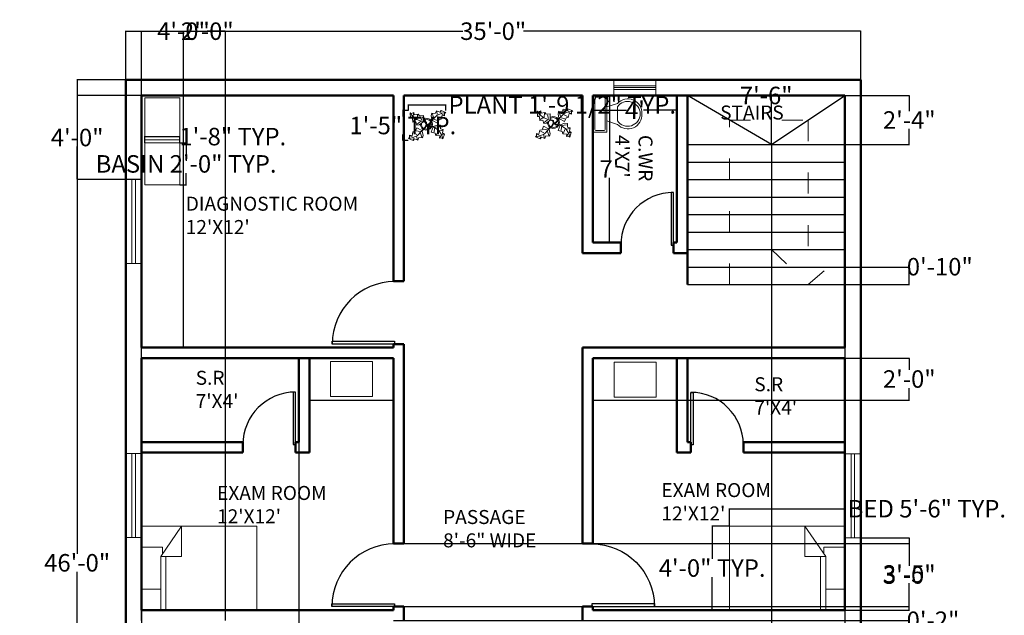
# Model space of a CAD drawing. Units: inches. Extents: x 69 to 644, y 258 to 887.
# Tile 3 of 3: x 82 to 644, y 546 to 887. Entities that reach past the tile are written whole.
import ezdxf

# ---------------------------------------------------------------- set-up
doc = ezdxf.new("R2010")
doc.units = ezdxf.units.IN
doc.header["$MEASUREMENT"] = 0
doc.linetypes.add('ACAD_ISO03W100', pattern=[30, 12, -18])
for name, color, linetype, lineweight in [('A-ANNO-DIMS', 2, 'Continuous', 18), ('A-AREA-IDEN', 7, 'Continuous', 25), ('A-DOOR', 4, 'Continuous', 25), ('A-EQPM-MED', 8, 'Continuous', 20), ('A-FLOR-CASE', 8, 'Continuous', 25), ('A-FLOR-FIXT', 9, 'Continuous', 18), ('A-FLOR-STRS', 7, 'Continuous', 25), ('A-FLOR-STRS-PATH', 7, 'ACAD_ISO03W100', 18), ('A-GLAZ', 4, 'Continuous', 18), ('A-WALL', 7, 'Continuous', 50), ('PLANT', 3, 'Continuous', 13)]:
    doc.layers.add(name, color=color, linetype=linetype, lineweight=lineweight)
doc.styles.get("Standard").update_dxf_attribs({"font": 'arial.ttf'})
doc.dimstyles.get("Standard").update_dxf_attribs({"dimtxt": 10, "dimasz": 0.18, "dimexe": 0.18, "dimexo": 0.0625, "dimgap": 0.09, "dimtad": 0, "dimtih": 1, "dimtoh": 1, "dimdec": 0, "dimzin": 0, "dimdsep": 46, "dimlunit": 3, "dimtxsty": 'Standard', "dimcen": 0.09, "dimadec": 0, "dimazin": 0, "dimtfac": 1, "dimtdec": 0, "dimtofl": 0, "dimtmove": 0, "dimatfit": 3, "dimfxl": 1, "dimtolj": 1, "dimtzin": 0, "dimarcsym": 0})

# ---------------------------------------------------------------- blocks, each defined once
blk = doc.blocks.new('SINGLE BED')
for p, q in [((0, 0), (0, -66)), ((48, 0), (0, 0)), ((12, 0), (12, -11)), ((36, -12), (36, 0)), ((48, -66), (48, 0)), ((0, -11), (30.52, -11)), ((30.52, -11), (48, -22.84)), ((30.52, -22.84), (30.52, -11)), ((0, -14), (30.52, -14)), ((31.99, -12), (36, -12)), ((48, -22.84), (30.52, -22.84)), ((0, -66), (48, -66))]:
    blk.add_line(p, q)
blk = doc.blocks.new('Plant - Rubber or Philodendron')
for p, q in [((-16.2005, 11.4774), (-13.9899, 8.1064)), ((-16.2005, 11.4774), (-14.8639, 10.7964)), ((-16.0159, 6.3329), (-16.2005, 11.4774)), ((-14.8639, 10.7964), (-12.6195, 11.8975)), ((-13.3174, 8.325), (-13.0735, 11.0065)), ((-12.6195, 11.8975), (-12.1909, 9.4345)), ((-12.1909, 9.4345), (-8.3829, 10.3)), ((-8.3829, 10.3), (-7.0549, 8.501)), ((4.6914, 8.8812), (5.3859, 11.2828)), ((5.3859, 11.2828), (8.8871, 10.7908)), ((5.9878, 10.4842), (7.1971, 6.3869)), ((8.8871, 10.7908), (9.9809, 13.4933)), ((9.9809, 13.4933), (13.3837, 12.301)), ((15.3859, 11.3055), (10.3916, 8.7942)), ((10.5828, 12.6946), (10.8893, 9.7953)), ((13.3837, 12.301), (14.68, 13.9039)), ((14.5816, 13.2037), (14.3848, 11.8033)), ((14.68, 13.9039), (19.3848, 11.8146)), ((15.2875, 10.6053), (17.5907, 9.2105)), ((19.3848, 11.8146), (15.3859, 11.3055)), ((19.3848, 11.8146), (18.1868, 10.9119)), ((18.1868, 10.9119), (18.1925, 8.4119)), ((-14.0069, 5.8704), (-16.0159, 6.3329)), ((-15.3434, 6.5514), (-13.9984, 6.9884)), ((-13.5868, 2.2894), (-14.0069, 5.8704)), ((-13.9899, 8.1064), (-9.5434, 4.7185)), ((-10.6784, 2.491), (-13.5868, 2.2894)), ((-13.1329, 3.1804), (-10.6614, 4.727)), ((-9.5858, -0.8715), (-10.6784, 2.491)), ((-9.5434, 4.7185), (-4.1917, 2.9888)), ((-9.1318, 0.0195), (-5.9793, 2.9025)), ((-8.8369, 9.409), (-9.0894, 5.6095)), ((-7.1228, -0.443), (-3.5248, 2.2131)), ((-7.0549, 8.501), (-3.0284, 8.6941)), ((-4.8529, 4.012), (-5.7184, 7.82)), ((-3.5248, 2.2131), (-3.3011, 2.4355)), ((-3.3011, 2.4355), (-0.5306, 1.7947)), ((-3.0284, 8.6941), (-3.0709, 3.1041)), ((-3.0709, 3.1041), (0.0797, 2.3163)), ((-0.5306, 1.7947), (-0.2255, -0.5527)), ((-0.5306, 1.7947), (-0.5306, 1.7947)), ((0.0797, 2.3163), (0.4866, -0.031)), ((0.4866, -0.031), (2.1141, 0.2298)), ((2.1141, 0.2298), (5.4346, 3.9146)), ((6.1032, 3.6844), (2.8262, -0.031)), ((4.6914, 8.8812), (5.5014, 4.4831)), ((5.4346, 3.9146), (5.5014, 4.4831)), ((11.1089, 1.1958), (6.1032, 3.6844)), ((10.3916, 8.7942), (6.2847, 4.4028)), ((7.7005, 4.8881), (11.5025, 3.9967)), ((14.2977, 6.1031), (10.9934, 7.9956)), ((12.7005, 4.8994), (11.1089, 1.1958)), ((14.8995, 5.3044), (12.7005, 4.8994)), ((15.7909, 9.1065), (14.8995, 5.3044)), ((18.1925, 8.4119), (15.7909, 9.1065)), ((-14.4141, -11.4699), (-13.5228, -7.6679)), ((-13.5228, -7.6679), (-11.3237, -7.2629)), ((-12.921, -8.4665), (-9.6166, -10.359)), ((-11.3237, -7.2629), (-9.7321, -3.5593)), ((-6.3237, -7.2516), (-10.1257, -6.3602)), ((-9.7321, -3.5593), (-4.7264, -6.0479)), ((-7.1228, -0.443), (-9.5858, -0.8715)), ((-9.0148, -11.1577), (-4.9047, -6.8122)), ((-4.611, -12.8477), (-5.8203, -8.7504)), ((-2.019, -3.6148), (-4.7264, -6.0479)), ((-4.1246, -6.8466), (-4.0579, -6.2781)), ((-3.3146, -11.2447), (-4.1246, -6.8466)), ((-4.0579, -6.2781), (-0.9375, -3.1608)), ((-2.019, -3.6148), (-0.2255, -0.5527)), ((-0.9375, -3.1608), (0.5883, -0.8135)), ((0.5883, -0.8135), (2.2447, -2.0916)), ((2.8262, -0.031), (1.3003, -0.5527)), ((1.3003, -0.5527), (2.4193, -1.4655)), ((2.2447, -2.0916), (6.7108, -2.6626)), ((2.4193, -1.4655), (6.895, -2.1175)), ((4.943, -7.9659), (6.7108, -2.6626)), ((8.8321, -9.0266), (4.943, -7.9659)), ((11.6605, -0.5413), (6.895, -2.1175)), ((12.3677, -6.1981), (7.219, -2.6772)), ((8.125, -4.0768), (7.7715, -7.9659)), ((8.3544, -2.7453), (13.1973, -2.1704)), ((9.5392, -11.1479), (8.8321, -9.0266)), ((10.2463, -10.4408), (11.6605, -6.9053)), ((11.6605, -0.5413), (14.1354, -0.8948)), ((15.5496, -10.7943), (12.3677, -6.1981)), ((16.2567, -5.8446), (13.4283, -6.5517)), ((14.1354, -0.8948), (14.1354, -4.4304)), ((14.1354, -4.4304), (16.9638, -5.1375)), ((17.3174, -9.7337), (15.9032, -9.7337)), ((16.9638, -5.1375), (16.2567, -8.673)), ((16.2567, -8.673), (18.0245, -9.7337)), ((18.0245, -9.7337), (16.6103, -14.6834)), ((-18.008, -14.1781), (-16.8101, -13.2754)), ((-18.008, -14.1781), (-14.0091, -13.669)), ((-13.3032, -16.2674), (-18.008, -14.1781)), ((-16.8157, -10.7754), (-14.4141, -11.4699)), ((-16.8101, -13.2754), (-16.8157, -10.7754)), ((-13.9107, -12.9688), (-16.2139, -11.574)), ((-14.0091, -13.669), (-9.0148, -11.1577)), ((-12.0069, -14.6645), (-13.3032, -16.2674)), ((-13.2048, -15.5672), (-13.008, -14.1668)), ((-8.6042, -15.8568), (-12.0069, -14.6645)), ((-9.206, -15.0581), (-9.5126, -12.1588)), ((-7.5103, -13.1543), (-8.6042, -15.8568)), ((-4.0092, -13.6463), (-7.5103, -13.1543)), ((-3.3146, -11.2447), (-4.0092, -13.6463)), ((13.4283, -11.5015), (9.5392, -11.1479)), ((13.0748, -13.9763), (13.4283, -11.5015)), ((15.5496, -13.6228), (13.0748, -13.9763)), ((14.8425, -10.7943), (13.7819, -13.2692)), ((16.6103, -14.6834), (15.5496, -10.7943)), ((16.6103, -14.6834), (15.5496, -13.6228))]:
    blk.add_line(p, q)
for centre, radius, start, end in [((0.0308, 0.1664), 6, 178.6147, 235.1169), ((0.0308, 0.1664), 5, 168.1647, 238.6725), ((0, 0), 6.1275, 34.37569, 120.1028), ((-0.0601, -0.2075), 5.2461, 33.82192, 124.9414), ((-0.2664, 0.1682), 5.2775, 338.4094, 20.03007), ((-0.098, 0.1364), 6.1288, 341.2017, 26.09184), ((-0.0234, 0.3825), 6.1492, 242.5812, 331.2714), ((-0.1102, 0.4886), 5.2883, 247.3711, 327.472)]:
    blk.add_arc(centre, radius, start, end)
blk = doc.blocks.new('*U14')
for p, q in [((0, 0), (0, -6)), ((40, 0), (40, -6))]:
    blk.add_line(p, q)
blk.add_lwpolyline([(0, 0), (0, 40), (1.75, 40), (1.75, 0)], close=True)
blk.add_arc((0, 0), 40, 0, 90)
blk = doc.blocks.new('*U15')
for p, q in [((0, 0), (0, -6)), ((-40, 0), (-40, -6))]:
    blk.add_line(p, q)
blk.add_lwpolyline([(0, 0), (0, 40), (-1.75, 40), (-1.75, 0)], close=True)
blk.add_arc((0, 0), 40, 90, 180)
blk = doc.blocks.new('*U17')
for p, q in [((9.5, -6), (9.5, -2)), ((-10, -8.5), (-8, -8.5)), ((-10, -9.5), (-10, -8.5)), ((-7, -9.5), (-10, -9.5)), ((-8, -8.5), (-8, -8)), ((-7, -8), (-7, -9.5)), ((-4, -8), (-6, -14)), ((4, -8), (6, -14)), ((4, -14), (-4, -14))]:
    blk.add_line(p, q)
blk.add_lwpolyline([(10.5, -8), (10.5, 0), (-10.5, 0), (-10.5, -8)], close=True)
for points in [[(-9.5, -2), (-9.5, -6)], [(8.5, -1), (-8.5, -1)], [(-8.5, -7), (8.5, -7)]]:
    blk.add_lwpolyline(points)
for centre, radius, start, end in [((-8.625, -1.875), 0.8839, 81.8699, 188.1301), ((8.625, -1.875), 0.8839, 351.8699, 98.1301), ((-8.625, -6.125), 0.8839, 171.869898, 278.1301), ((8.625, -6.125), 0.8839, 261.8699, 8.1301), ((-0.4772, -19.9188), 8.0953, 133.01722, 273.38), ((0.0374, -19.8731), 7.127, 124.50543, 269.7), ((-0.0373, -19.8731), 7.127, 270.3, 55.4946), ((0.4773, -19.9188), 8.0953, 266.62, 46.9828)]:
    blk.add_arc(centre, radius, start, end)
blk = doc.blocks.new('*D20')
at = {"layer": 'A-ANNO-DIMS', "color": 0, "lineweight": -2, "transparency": 16777216}
for p, q in [((409.27, 843.36), (409.27, 834.9)), ((457.27, 843.36), (457.27, 834.9)), ((409.45, 835.08), (428.37, 835.08)), ((457.09, 835.08), (438.16, 835.08))]:
    blk.add_line(p, q, dxfattribs=at)
at = {"layer": 'A-ANNO-DIMS', "color": 0, "transparency": 16777216}
for points in [[(409.45, 835.11), (409.45, 835.05), (409.27, 835.08)], [(457.09, 835.11), (457.09, 835.05), (457.27, 835.08)]]:
    blk.add_solid(points, dxfattribs=at)
at = {"layer": 'Defpoints', "color": 0, "transparency": 16777216}
for p in [(409.27, 843.42), (457.27, 843.42), (457.27, 835.08)]:
    blk.add_point(p, dxfattribs=at)
at = {"layer": 'A-ANNO-DIMS', "color": 0, "transparency": 16777216, "insert": (433.27, 835.08), "char_height": 10, "attachment_point": 5}
blk.add_mtext("\\A1;4'", dxfattribs=at)
blk = doc.blocks.new('*D21')
at = {"layer": 'A-ANNO-DIMS', "color": 0, "lineweight": -2, "transparency": 16777216}
for p, q in [((409.33, 843.42), (418.84, 843.42)), ((418.66, 843.24), (418.66, 806.51)), ((418.66, 759.6), (418.66, 796.33)), ((409.33, 759.42), (418.84, 759.42))]:
    blk.add_line(p, q, dxfattribs=at)
at = {"layer": 'A-ANNO-DIMS', "color": 0, "transparency": 16777216}
for points in [[(418.63, 843.24), (418.69, 843.24), (418.66, 843.42)], [(418.63, 759.6), (418.69, 759.6), (418.66, 759.42)]]:
    blk.add_solid(points, dxfattribs=at)
at = {"layer": 'Defpoints', "color": 0, "transparency": 16777216}
for p in [(409.27, 843.42), (409.27, 759.42), (418.66, 759.42)]:
    blk.add_point(p, dxfattribs=at)
at = {"layer": 'A-ANNO-DIMS', "color": 0, "transparency": 16777216, "insert": (418.66, 801.42), "char_height": 10, "attachment_point": 5}
blk.add_mtext("\\A1;7'", dxfattribs=at)
blk = doc.blocks.new('*D22')
at = {"layer": 'A-ANNO-DIMS', "color": 0, "lineweight": -2, "transparency": 16777216}
for p, q in [((463.27, 843.36), (463.27, 843.24)), ((463.45, 843.42), (494.93, 843.42)), ((553.09, 843.42), (521.61, 843.42)), ((553.27, 843.36), (553.27, 843.24))]:
    blk.add_line(p, q, dxfattribs=at)
at = {"layer": 'A-ANNO-DIMS', "color": 0, "transparency": 16777216}
for points in [[(463.45, 843.45), (463.45, 843.39), (463.27, 843.42)], [(553.09, 843.45), (553.09, 843.39), (553.27, 843.42)]]:
    blk.add_solid(points, dxfattribs=at)
at = {"layer": 'Defpoints', "color": 0, "transparency": 16777216}
for p in [(463.27, 843.42), (553.27, 843.42), (553.27, 843.42)]:
    blk.add_point(p, dxfattribs=at)
at = {"layer": 'A-ANNO-DIMS', "color": 0, "transparency": 16777216, "insert": (508.27, 843.42), "char_height": 10, "attachment_point": 5}
blk.add_mtext('\\A1;7\'-6"', dxfattribs=at)
blk = doc.blocks.new('WIN-48IN')
for p, q in [((9, 48), (0, 48)), ((3.5, 0), (3.5, 48)), ((5.5, 0), (5.5, 48)), ((9, 0), (0, 0))]:
    blk.add_line(p, q)
blk = doc.blocks.new('WIN-24IN')
for p, q in [((0, 0), (0, 9)), ((24, 0), (24, 9)), ((0, 5.5), (24, 5.5)), ((0, 4.5), (24, 4.5)), ((0, 3.5), (24, 3.5))]:
    blk.add_line(p, q)
blk = doc.blocks.new('COUNTER-BASIN-24X20')
for p, q in [((0, 20), (24, 20)), ((0, 0), (0, 20)), ((24, 0), (24, 20)), ((0, 0), (24, 0))]:
    blk.add_line(p, q)
blk = doc.blocks.new('*D29')
at = {"layer": 'A-ANNO-DIMS', "color": 0, "lineweight": -2, "transparency": 16777216}
for p, q in [((303.83, 834.94), (303.83, 838.25)), ((304.01, 838.07), (324.96, 838.07)), ((325.14, 834.94), (325.14, 838.25)), ((325.14, 838.07), (325.32, 838.07))]:
    blk.add_line(p, q, dxfattribs=at)
at = {"layer": 'A-ANNO-DIMS', "color": 0, "transparency": 16777216}
for points in [[(304.01, 838.1), (304.01, 838.04), (303.83, 838.07)], [(324.96, 838.1), (324.96, 838.04), (325.14, 838.07)]]:
    blk.add_solid(points, dxfattribs=at)
at = {"layer": 'Defpoints', "color": 0, "transparency": 16777216}
for p in [(303.83, 834.87), (325.14, 838.07), (325.14, 834.87)]:
    blk.add_point(p, dxfattribs=at)
at = {"layer": 'A-ANNO-DIMS', "color": 0, "transparency": 16777216, "insert": (391.74, 838.07), "char_height": 10, "attachment_point": 5}
blk.add_mtext('\\A1;PLANT 1\'-9 1/2" TYP.', dxfattribs=at)
blk = doc.blocks.new('*D30')
at = {"layer": 'A-ANNO-DIMS', "color": 0, "lineweight": -2, "transparency": 16777216}
for p, q in [((303.77, 834.87), (300.45, 834.87)), ((300.63, 834.69), (300.63, 831.47)), ((303.77, 817.68), (300.45, 817.68)), ((300.63, 817.86), (300.63, 821.08))]:
    blk.add_line(p, q, dxfattribs=at)
at = {"layer": 'A-ANNO-DIMS', "color": 0, "transparency": 16777216}
for points in [[(300.6, 834.69), (300.66, 834.69), (300.63, 834.87)], [(300.6, 817.86), (300.66, 817.86), (300.63, 817.68)]]:
    blk.add_solid(points, dxfattribs=at)
at = {"layer": 'Defpoints', "color": 0, "transparency": 16777216}
for p in [(300.63, 834.87), (303.83, 834.87), (303.83, 817.68)]:
    blk.add_point(p, dxfattribs=at)
at = {"layer": 'A-ANNO-DIMS', "color": 0, "transparency": 16777216, "insert": (300.63, 826.28), "char_height": 10, "attachment_point": 5}
blk.add_mtext('\\A1;1\'-5" TYP.', dxfattribs=at)
blk = doc.blocks.new('*D33')
at = {"layer": 'A-ANNO-DIMS', "color": 0, "lineweight": -2, "transparency": 16777216}
for p, q in [((151.33, 532.77), (155.05, 532.77)), ((154.87, 532.59), (154.87, 526.03)), ((154.87, 508.95), (154.87, 515.5)), ((151.33, 508.77), (155.05, 508.77))]:
    blk.add_line(p, q, dxfattribs=at)
at = {"layer": 'A-ANNO-DIMS', "color": 0, "transparency": 16777216}
for points in [[(154.84, 532.59), (154.9, 532.59), (154.87, 532.77)], [(154.84, 508.95), (154.9, 508.95), (154.87, 508.77)]]:
    blk.add_solid(points, dxfattribs=at)
at = {"layer": 'Defpoints', "color": 0, "transparency": 16777216}
for p in [(151.27, 532.77), (154.87, 532.77), (151.27, 508.77)]:
    blk.add_point(p, dxfattribs=at)
at = {"layer": 'A-ANNO-DIMS', "color": 0, "transparency": 16777216, "insert": (154.87, 520.77), "char_height": 10, "attachment_point": 5}
blk.add_mtext('\\A1;WINDOW B 2\'-0" TYP.', dxfattribs=at)
blk = doc.blocks.new('*D34')
at = {"layer": 'A-ANNO-DIMS', "color": 0, "lineweight": -2, "transparency": 16777216}
for p, q in [((142.27, 536.37), (142.09, 536.37)), ((142.27, 532.83), (142.27, 536.55)), ((151.09, 536.37), (142.45, 536.37)), ((151.27, 532.83), (151.27, 536.55))]:
    blk.add_line(p, q, dxfattribs=at)
at = {"layer": 'A-ANNO-DIMS', "color": 0, "transparency": 16777216}
for points in [[(142.45, 536.4), (142.45, 536.34), (142.27, 536.37)], [(151.09, 536.4), (151.09, 536.34), (151.27, 536.37)]]:
    blk.add_solid(points, dxfattribs=at)
at = {"layer": 'Defpoints', "color": 0, "transparency": 16777216}
for p in [(142.27, 536.37), (142.27, 532.77), (151.27, 532.77)]:
    blk.add_point(p, dxfattribs=at)
at = {"layer": 'A-ANNO-DIMS', "color": 0, "transparency": 16777216, "insert": (111.52, 536.37), "char_height": 10, "attachment_point": 5}
blk.add_mtext('\\A1;0\'-9" TYP.', dxfattribs=at)
blk = doc.blocks.new('*D37')
at = {"layer": 'A-ANNO-DIMS', "color": 0, "lineweight": -2, "transparency": 16777216}
for p, q in [((173.25, 816.34), (176.97, 816.34)), ((176.79, 816.16), (176.79, 809.6)), ((176.79, 792.52), (176.79, 799.08)), ((173.25, 792.34), (176.97, 792.34))]:
    blk.add_line(p, q, dxfattribs=at)
at = {"layer": 'A-ANNO-DIMS', "color": 0, "transparency": 16777216}
for points in [[(176.76, 816.16), (176.82, 816.16), (176.79, 816.34)], [(176.76, 792.52), (176.82, 792.52), (176.79, 792.34)]]:
    blk.add_solid(points, dxfattribs=at)
at = {"layer": 'Defpoints', "color": 0, "transparency": 16777216}
for p in [(173.19, 816.34), (173.19, 792.34), (176.79, 792.34)]:
    blk.add_point(p, dxfattribs=at)
at = {"layer": 'A-ANNO-DIMS', "color": 0, "transparency": 16777216, "insert": (176.79, 804.34), "char_height": 10, "attachment_point": 5}
blk.add_mtext('\\A1;BASIN 2\'-0" TYP.', dxfattribs=at)
blk = doc.blocks.new('*D38')
at = {"layer": 'A-ANNO-DIMS', "color": 0, "lineweight": -2, "transparency": 16777216}
for p, q in [((153.19, 816.41), (153.19, 820.12)), ((153.37, 819.94), (173.01, 819.94)), ((173.19, 816.41), (173.19, 820.12)), ((173.19, 819.94), (173.37, 819.94))]:
    blk.add_line(p, q, dxfattribs=at)
at = {"layer": 'A-ANNO-DIMS', "color": 0, "transparency": 16777216}
for points in [[(153.37, 819.97), (153.37, 819.91), (153.19, 819.94)], [(173.01, 819.97), (173.01, 819.91), (173.19, 819.94)]]:
    blk.add_solid(points, dxfattribs=at)
at = {"layer": 'Defpoints', "color": 0, "transparency": 16777216}
for p in [(153.19, 816.34), (173.19, 819.94), (173.19, 816.34)]:
    blk.add_point(p, dxfattribs=at)
at = {"layer": 'A-ANNO-DIMS', "color": 0, "transparency": 16777216, "insert": (203.47, 819.94), "char_height": 10, "attachment_point": 5}
blk.add_mtext('\\A1;1\'-8" TYP.', dxfattribs=at)
blk = doc.blocks.new('*D49')
at = {"layer": 'A-ANNO-DIMS', "color": 0, "lineweight": -2, "transparency": 16777216}
for p, q in [((487.27, 597.48), (487.27, 607.5)), ((487.45, 607.32), (553.09, 607.32)), ((553.27, 597.48), (553.27, 607.5)), ((553.27, 607.32), (553.45, 607.32))]:
    blk.add_line(p, q, dxfattribs=at)
at = {"layer": 'A-ANNO-DIMS', "color": 0, "transparency": 16777216}
for points in [[(487.45, 607.35), (487.45, 607.29), (487.27, 607.32)], [(553.09, 607.35), (553.09, 607.29), (553.27, 607.32)]]:
    blk.add_solid(points, dxfattribs=at)
at = {"layer": 'Defpoints', "color": 0, "transparency": 16777216}
for p in [(553.27, 607.32), (487.27, 597.42), (553.27, 597.42)]:
    blk.add_point(p, dxfattribs=at)
at = {"layer": 'A-ANNO-DIMS', "color": 0, "transparency": 16777216, "insert": (600.09, 607.32), "char_height": 10, "attachment_point": 5}
blk.add_mtext('\\A1;BED 5\'-6" TYP.', dxfattribs=at)
blk = doc.blocks.new('*D50')
at = {"layer": 'A-ANNO-DIMS', "color": 0, "lineweight": -2, "transparency": 16777216}
for p, q in [((487.2, 597.42), (477.19, 597.42)), ((477.37, 597.24), (477.37, 578.62)), ((477.37, 549.6), (477.37, 568.22)), ((487.2, 549.42), (477.19, 549.42))]:
    blk.add_line(p, q, dxfattribs=at)
at = {"layer": 'A-ANNO-DIMS', "color": 0, "transparency": 16777216}
for points in [[(477.34, 597.24), (477.4, 597.24), (477.37, 597.42)], [(477.34, 549.6), (477.4, 549.6), (477.37, 549.42)]]:
    blk.add_solid(points, dxfattribs=at)
at = {"layer": 'Defpoints', "color": 0, "transparency": 16777216}
for p in [(477.37, 597.42), (487.27, 597.42), (487.27, 549.42)]:
    blk.add_point(p, dxfattribs=at)
at = {"layer": 'A-ANNO-DIMS', "color": 0, "transparency": 16777216, "insert": (477.37, 573.42), "char_height": 10, "attachment_point": 5}
blk.add_mtext('\\A1;4\'-0" TYP.', dxfattribs=at)
blk = doc.blocks.new('*D51')
at = {"layer": 'A-ANNO-DIMS', "color": 0, "lineweight": -2, "transparency": 16777216}
for p, q in [((142.27, 852.48), (142.27, 880.35)), ((142.45, 880.17), (335, 880.17)), ((562.09, 880.17), (369.53, 880.17)), ((562.27, 852.48), (562.27, 880.35))]:
    blk.add_line(p, q, dxfattribs=at)
at = {"layer": 'A-ANNO-DIMS', "color": 0, "transparency": 16777216}
for points in [[(142.45, 880.2), (142.45, 880.14), (142.27, 880.17)], [(562.09, 880.2), (562.09, 880.14), (562.27, 880.17)]]:
    blk.add_solid(points, dxfattribs=at)
at = {"layer": 'Defpoints', "color": 0, "transparency": 16777216}
for p in [(562.27, 880.17), (142.27, 852.42), (562.27, 852.42)]:
    blk.add_point(p, dxfattribs=at)
at = {"layer": 'A-ANNO-DIMS', "color": 0, "transparency": 16777216, "insert": (352.27, 880.17), "char_height": 10, "attachment_point": 5}
blk.add_mtext('\\A1;35\'-0"', dxfattribs=at)
blk = doc.blocks.new('*D52')
at = {"layer": 'A-ANNO-DIMS', "color": 0, "lineweight": -2, "transparency": 16777216}
for p, q in [((142.2, 852.42), (114.34, 852.42)), ((114.52, 852.24), (114.52, 581.62)), ((114.52, 300.6), (114.52, 571.22)), ((142.2, 300.42), (114.34, 300.42))]:
    blk.add_line(p, q, dxfattribs=at)
at = {"layer": 'A-ANNO-DIMS', "color": 0, "transparency": 16777216}
for points in [[(114.49, 852.24), (114.55, 852.24), (114.52, 852.42)], [(114.49, 300.6), (114.55, 300.6), (114.52, 300.42)]]:
    blk.add_solid(points, dxfattribs=at)
at = {"layer": 'Defpoints', "color": 0, "transparency": 16777216}
for p in [(114.52, 852.42), (142.27, 852.42), (142.27, 300.42)]:
    blk.add_point(p, dxfattribs=at)
at = {"layer": 'A-ANNO-DIMS', "color": 0, "transparency": 16777216, "insert": (114.52, 576.42), "char_height": 10, "attachment_point": 5}
blk.add_mtext('\\A1;46\'-0"', dxfattribs=at)
blk = doc.blocks.new('*D57')
at = {"layer": 'A-ANNO-DIMS', "color": 0, "lineweight": -2, "transparency": 16777216}
for p, q in [((295.33, 587.42), (590.2, 587.42)), ((590.02, 587.24), (590.02, 574.62)), ((590.02, 551.6), (590.02, 564.22)), ((295.33, 551.42), (590.2, 551.42))]:
    blk.add_line(p, q, dxfattribs=at)
at = {"layer": 'A-ANNO-DIMS', "color": 0, "transparency": 16777216}
for points in [[(589.99, 587.24), (590.05, 587.24), (590.02, 587.42)], [(589.99, 551.6), (590.05, 551.6), (590.02, 551.42)]]:
    blk.add_solid(points, dxfattribs=at)
at = {"layer": 'Defpoints', "color": 0, "transparency": 16777216}
for p in [(295.27, 587.42), (295.27, 551.42), (590.02, 551.42)]:
    blk.add_point(p, dxfattribs=at)
at = {"layer": 'A-ANNO-DIMS', "color": 0, "transparency": 16777216, "insert": (590.02, 569.42), "char_height": 10, "attachment_point": 5}
blk.add_mtext('\\A1;3\'-0"', dxfattribs=at)
blk = doc.blocks.new('*D59')
at = {"layer": 'A-ANNO-DIMS', "color": 0, "lineweight": -2, "transparency": 16777216}
for p, q in [((151.27, 543.48), (151.27, 880.35)), ((151.45, 880.17), (161.68, 880.17)), ((199.09, 880.17), (188.85, 880.17)), ((199.27, 543.48), (199.27, 880.35))]:
    blk.add_line(p, q, dxfattribs=at)
at = {"layer": 'A-ANNO-DIMS', "color": 0, "transparency": 16777216}
for points in [[(151.45, 880.2), (151.45, 880.14), (151.27, 880.17)], [(199.09, 880.2), (199.09, 880.14), (199.27, 880.17)]]:
    blk.add_solid(points, dxfattribs=at)
at = {"layer": 'Defpoints', "color": 0, "transparency": 16777216}
for p in [(199.27, 880.17), (151.27, 543.42), (199.27, 543.42)]:
    blk.add_point(p, dxfattribs=at)
at = {"layer": 'A-ANNO-DIMS', "color": 0, "transparency": 16777216, "insert": (175.27, 880.17), "char_height": 10, "attachment_point": 5}
blk.add_mtext('\\A1;4\'-0"', dxfattribs=at)
blk = doc.blocks.new('*D64')
at = {"layer": 'A-ANNO-DIMS', "color": 0, "lineweight": -2, "transparency": 16777216}
for p, q in [((553.33, 843.42), (590.2, 843.42)), ((590.02, 843.24), (590.02, 834.53)), ((590.02, 815.6), (590.02, 824.31)), ((553.33, 815.42), (590.2, 815.42))]:
    blk.add_line(p, q, dxfattribs=at)
at = {"layer": 'A-ANNO-DIMS', "color": 0, "transparency": 16777216}
for points in [[(589.99, 843.24), (590.05, 843.24), (590.02, 843.42)], [(589.99, 815.6), (590.05, 815.6), (590.02, 815.42)]]:
    blk.add_solid(points, dxfattribs=at)
at = {"layer": 'Defpoints', "color": 0, "transparency": 16777216}
for p in [(553.27, 843.42), (553.27, 815.42), (590.02, 815.42)]:
    blk.add_point(p, dxfattribs=at)
at = {"layer": 'A-ANNO-DIMS', "color": 0, "transparency": 16777216, "insert": (590.02, 829.42), "char_height": 10, "attachment_point": 5}
blk.add_mtext('\\A1;2\'-4"', dxfattribs=at)
blk = doc.blocks.new('*D65')
at = {"layer": 'A-ANNO-DIMS', "color": 0, "lineweight": -2, "transparency": 16777216}
for p, q in [((553.33, 745.42), (590.2, 745.42)), ((590.02, 745.42), (590.02, 745.6)), ((590.02, 745.6), (590.2, 745.6)), ((590.02, 735.6), (590.02, 745.24)), ((553.33, 735.42), (590.2, 735.42))]:
    blk.add_line(p, q, dxfattribs=at)
at = {"layer": 'A-ANNO-DIMS', "color": 0, "transparency": 16777216}
for points in [[(589.99, 745.24), (590.05, 745.24), (590.02, 745.42)], [(589.99, 735.6), (590.05, 735.6), (590.02, 735.42)]]:
    blk.add_solid(points, dxfattribs=at)
at = {"layer": 'Defpoints', "color": 0, "transparency": 16777216}
for p in [(553.27, 745.42), (590.02, 745.42), (553.27, 735.42)]:
    blk.add_point(p, dxfattribs=at)
at = {"layer": 'A-ANNO-DIMS', "color": 0, "transparency": 16777216, "insert": (607.46, 745.6), "char_height": 10, "attachment_point": 5}
blk.add_mtext('\\A1;0\'-10"', dxfattribs=at)
blk = doc.blocks.new('*D66')
at = {"layer": 'A-ANNO-DIMS', "color": 0, "lineweight": -2, "transparency": 16777216}
for p, q in [((511.27, 735.36), (511.27, 272.49)), ((553.27, 735.36), (553.27, 272.49)), ((511.45, 272.67), (518.89, 272.67)), ((553.09, 272.67), (545.64, 272.67))]:
    blk.add_line(p, q, dxfattribs=at)
at = {"layer": 'A-ANNO-DIMS', "color": 0, "transparency": 16777216}
for points in [[(511.45, 272.7), (511.45, 272.64), (511.27, 272.67)], [(553.09, 272.7), (553.09, 272.64), (553.27, 272.67)]]:
    blk.add_solid(points, dxfattribs=at)
at = {"layer": 'Defpoints', "color": 0, "transparency": 16777216}
for p in [(511.27, 735.42), (553.27, 735.42), (553.27, 272.67)]:
    blk.add_point(p, dxfattribs=at)
at = {"layer": 'A-ANNO-DIMS', "color": 0, "transparency": 16777216, "insert": (532.27, 272.67), "char_height": 10, "attachment_point": 5}
blk.add_mtext('\\A1;3\'-6"', dxfattribs=at)
blk = doc.blocks.new('*D67')
at = {"layer": 'A-ANNO-DIMS', "color": 0, "lineweight": -2, "transparency": 16777216}
for p, q in [((562.33, 590.65), (590.2, 590.65)), ((590.02, 590.47), (590.02, 575.24)), ((590.02, 549.6), (590.02, 564.84)), ((553.33, 549.42), (590.2, 549.42))]:
    blk.add_line(p, q, dxfattribs=at)
at = {"layer": 'A-ANNO-DIMS', "color": 0, "transparency": 16777216}
for points in [[(589.99, 590.47), (590.05, 590.47), (590.02, 590.65)], [(589.99, 549.6), (590.05, 549.6), (590.02, 549.42)]]:
    blk.add_solid(points, dxfattribs=at)
at = {"layer": 'Defpoints', "color": 0, "transparency": 16777216}
for p in [(562.27, 590.65), (590.02, 590.65), (553.27, 549.42)]:
    blk.add_point(p, dxfattribs=at)
at = {"layer": 'A-ANNO-DIMS', "color": 0, "transparency": 16777216, "insert": (590.02, 570.04), "char_height": 10, "attachment_point": 5}
blk.add_mtext('\\A1;3\'-5"', dxfattribs=at)
blk = doc.blocks.new('*D68')
at = {"layer": 'A-ANNO-DIMS', "color": 0, "lineweight": -2, "transparency": 16777216}
for p, q in [((151.2, 843.42), (114.34, 843.42)), ((114.52, 843.24), (114.52, 824.62)), ((114.52, 795.6), (114.52, 814.22)), ((151.2, 795.42), (114.34, 795.42))]:
    blk.add_line(p, q, dxfattribs=at)
at = {"layer": 'A-ANNO-DIMS', "color": 0, "transparency": 16777216}
for points in [[(114.49, 843.24), (114.55, 843.24), (114.52, 843.42)], [(114.49, 795.6), (114.55, 795.6), (114.52, 795.42)]]:
    blk.add_solid(points, dxfattribs=at)
at = {"layer": 'Defpoints', "color": 0, "transparency": 16777216}
for p in [(151.27, 843.42), (114.52, 795.42), (151.27, 795.42)]:
    blk.add_point(p, dxfattribs=at)
at = {"layer": 'A-ANNO-DIMS', "color": 0, "transparency": 16777216, "insert": (114.52, 819.42), "char_height": 10, "attachment_point": 5}
blk.add_mtext('\\A1;4\'-0"', dxfattribs=at)
blk = doc.blocks.new('*D69')
at = {"layer": 'A-ANNO-DIMS', "color": 0, "lineweight": -2, "transparency": 16777216}
for p, q in [((151.27, 693.36), (151.27, 272.49)), ((241.27, 693.36), (241.27, 272.49)), ((151.45, 272.67), (182.93, 272.67)), ((241.09, 272.67), (209.61, 272.67))]:
    blk.add_line(p, q, dxfattribs=at)
at = {"layer": 'A-ANNO-DIMS', "color": 0, "transparency": 16777216}
for points in [[(151.45, 272.7), (151.45, 272.64), (151.27, 272.67)], [(241.09, 272.7), (241.09, 272.64), (241.27, 272.67)]]:
    blk.add_solid(points, dxfattribs=at)
at = {"layer": 'Defpoints', "color": 0, "transparency": 16777216}
for p in [(151.27, 693.42), (241.27, 693.42), (241.27, 272.67)]:
    blk.add_point(p, dxfattribs=at)
at = {"layer": 'A-ANNO-DIMS', "color": 0, "transparency": 16777216, "insert": (196.27, 272.67), "char_height": 10, "attachment_point": 5}
blk.add_mtext('\\A1;7\'-6"', dxfattribs=at)
blk = doc.blocks.new('*D70')
at = {"layer": 'A-ANNO-DIMS', "color": 0, "lineweight": -2, "transparency": 16777216}
for p, q in [((295.33, 543.42), (590.2, 543.42)), ((295.33, 541.42), (590.2, 541.42)), ((590.02, 543.42), (590.02, 543.6)), ((590.02, 543.6), (590.2, 543.6)), ((590.02, 541.6), (590.02, 543.24))]:
    blk.add_line(p, q, dxfattribs=at)
at = {"layer": 'A-ANNO-DIMS', "color": 0, "transparency": 16777216}
for points in [[(589.99, 543.24), (590.05, 543.24), (590.02, 543.42)], [(589.99, 541.6), (590.05, 541.6), (590.02, 541.42)]]:
    blk.add_solid(points, dxfattribs=at)
at = {"layer": 'Defpoints', "color": 0, "transparency": 16777216}
for p in [(295.27, 543.42), (295.27, 541.42), (590.02, 543.42)]:
    blk.add_point(p, dxfattribs=at)
at = {"layer": 'A-ANNO-DIMS', "color": 0, "transparency": 16777216, "insert": (603.58, 543.6), "char_height": 10, "attachment_point": 5}
blk.add_mtext('\\A1;0\'-2"', dxfattribs=at)
blk = doc.blocks.new('*D73')
at = {"layer": 'A-ANNO-DIMS', "color": 0, "lineweight": -2, "transparency": 16777216}
for p, q in [((151.27, 843.48), (151.27, 880.35)), ((151.45, 880.17), (175.09, 880.17)), ((175.27, 843.48), (175.27, 880.35)), ((175.27, 880.17), (175.45, 880.17))]:
    blk.add_line(p, q, dxfattribs=at)
at = {"layer": 'A-ANNO-DIMS', "color": 0, "transparency": 16777216}
for points in [[(151.45, 880.2), (151.45, 880.14), (151.27, 880.17)], [(175.09, 880.2), (175.09, 880.14), (175.27, 880.17)]]:
    blk.add_solid(points, dxfattribs=at)
at = {"layer": 'Defpoints', "color": 0, "transparency": 16777216}
for p in [(175.27, 880.17), (151.27, 843.42), (175.27, 843.42)]:
    blk.add_point(p, dxfattribs=at)
at = {"layer": 'A-ANNO-DIMS', "color": 0, "transparency": 16777216, "insert": (188.91, 880.17), "char_height": 10, "attachment_point": 5}
blk.add_mtext('\\A1;2\'-0"', dxfattribs=at)
blk = doc.blocks.new('*D74')
at = {"layer": 'A-ANNO-DIMS', "color": 0, "lineweight": -2, "transparency": 16777216}
for p, q in [((409.33, 693.42), (590.2, 693.42)), ((590.02, 693.24), (590.02, 686.62)), ((590.02, 669.6), (590.02, 676.22)), ((409.33, 669.42), (590.2, 669.42))]:
    blk.add_line(p, q, dxfattribs=at)
at = {"layer": 'A-ANNO-DIMS', "color": 0, "transparency": 16777216}
for points in [[(589.99, 693.24), (590.05, 693.24), (590.02, 693.42)], [(589.99, 669.6), (590.05, 669.6), (590.02, 669.42)]]:
    blk.add_solid(points, dxfattribs=at)
at = {"layer": 'Defpoints', "color": 0, "transparency": 16777216}
for p in [(409.27, 693.42), (409.27, 669.42), (590.02, 669.42)]:
    blk.add_point(p, dxfattribs=at)
at = {"layer": 'A-ANNO-DIMS', "color": 0, "transparency": 16777216, "insert": (590.02, 681.42), "char_height": 10, "attachment_point": 5}
blk.add_mtext('\\A1;2\'-0"', dxfattribs=at)

msp = doc.modelspace()

# ---------------------------------------------------------------- linework, layer by layer
at = {"layer": 'A-FLOR-CASE'}
for p, q in [((175.27, 699.42), (175.27, 843.42)), ((247.27, 669.42), (295.27, 669.42)), ((409.27, 669.42), (457.27, 669.42))]:
    msp.add_line(p, q, dxfattribs=at)
at = {"layer": 'A-FLOR-STRS'}
for p, q in [((511.27, 815.42), (463.27, 843.42)), ((511.27, 815.42), (511.27, 843.42)), ((511.27, 815.42), (553.27, 843.42)), ((463.27, 815.42), (553.27, 815.42)), ((511.27, 815.42), (511.27, 735.42)), ((463.27, 805.42), (553.27, 805.42)), ((463.27, 795.42), (553.27, 795.42)), ((463.27, 785.42), (553.27, 785.42)), ((463.27, 775.42), (553.27, 775.42)), ((463.27, 765.42), (553.27, 765.42)), ((463.27, 755.42), (553.27, 755.42)), ((463.27, 745.42), (553.27, 745.42)), ((463.27, 735.42), (553.27, 735.42)), ((463.27, 735.42), (511.27, 735.42)), ((511.27, 735.42), (553.27, 735.42))]:
    msp.add_line(p, q, dxfattribs=at)
at = {"layer": 'A-FLOR-STRS-PATH'}
for p, q in [((487.27, 735.42), (487.27, 829.42)), ((487.27, 829.42), (532.27, 829.42)), ((532.27, 829.42), (532.27, 755.42)), ((532.27, 755.42), (511.27, 755.42)), ((511.27, 755.42), (532.27, 735.42)), ((532.27, 755.42), (553.27, 755.42)), ((532.27, 735.42), (553.27, 753.42))]:
    msp.add_line(p, q, dxfattribs=at)
at = {"layer": 'A-WALL'}
for p, q in [((142.27, 300.42), (142.27, 852.42)), ((142.27, 852.42), (562.27, 852.42)), ((562.27, 852.42), (562.27, 300.42)), ((151.27, 843.42), (295.27, 843.42)), ((151.27, 699.42), (151.27, 843.42)), ((295.27, 737.42), (295.27, 843.42)), ((301.27, 843.42), (403.27, 843.42)), ((301.27, 737.42), (301.27, 843.42)), ((403.27, 843.42), (403.27, 753.42)), ((409.27, 843.42), (409.27, 759.42)), ((409.27, 843.42), (553.27, 843.42)), ((409.27, 843.42), (457.27, 843.42)), ((457.27, 843.42), (457.27, 759.42)), ((463.27, 843.42), (463.27, 735.42)), ((553.27, 843.42), (553.27, 753.42)), ((409.27, 759.42), (425.27, 759.42)), ((425.27, 759.42), (425.27, 753.42)), ((455.27, 753.42), (455.27, 759.42)), ((455.27, 759.42), (457.27, 759.42)), ((403.27, 753.42), (425.27, 753.42)), ((457.27, 753.42), (455.27, 753.42)), ((457.27, 753.42), (463.27, 753.42)), ((553.27, 753.42), (553.27, 699.42)), ((295.27, 737.42), (301.27, 737.42)), ((151.27, 699.42), (295.27, 699.42)), ((301.27, 701.42), (295.27, 701.42)), ((295.27, 701.42), (295.27, 699.42)), ((301.27, 699.42), (301.27, 701.42)), ((301.27, 587.42), (301.27, 699.42)), ((403.27, 699.42), (553.27, 699.42)), ((403.27, 699.42), (403.27, 587.42)), ((151.27, 693.42), (295.27, 693.42)), ((151.27, 549.42), (151.27, 693.42)), ((241.27, 645.42), (241.27, 693.42)), ((247.27, 639.42), (247.27, 693.42)), ((295.27, 587.42), (295.27, 693.42)), ((409.27, 693.42), (553.27, 693.42)), ((409.27, 693.42), (409.27, 587.42)), ((457.27, 693.42), (457.27, 639.42)), ((463.27, 693.42), (463.27, 645.42)), ((553.27, 693.42), (553.27, 549.42)), ((151.27, 645.42), (209.27, 645.42)), ((209.27, 639.42), (209.27, 645.42)), ((239.27, 639.42), (239.27, 645.42)), ((239.27, 645.42), (241.27, 645.42)), ((465.27, 645.42), (463.27, 645.42)), ((465.27, 639.42), (465.27, 645.42)), ((495.27, 645.42), (553.27, 645.42)), ((495.27, 645.42), (495.27, 639.42)), ((151.27, 639.42), (209.27, 639.42)), ((241.27, 639.42), (239.27, 639.42)), ((241.27, 639.42), (247.27, 639.42)), ((457.27, 639.42), (463.27, 639.42)), ((463.27, 639.42), (465.27, 639.42)), ((495.27, 639.42), (553.27, 639.42)), ((295.27, 587.42), (301.27, 587.42)), ((403.27, 587.42), (409.27, 587.42)), ((301.27, 551.42), (295.27, 551.42)), ((295.27, 551.42), (295.27, 549.42)), ((301.27, 549.42), (301.27, 551.42)), ((403.27, 549.42), (403.27, 551.42)), ((403.27, 551.42), (409.27, 551.42)), ((409.27, 551.42), (409.27, 549.42)), ((151.27, 549.42), (295.27, 549.42)), ((301.27, 543.42), (301.27, 549.42)), ((403.27, 549.42), (403.27, 543.42)), ((409.27, 549.42), (553.27, 549.42))]:
    msp.add_line(p, q, dxfattribs=at)

# ---------------------------------------------------------------- block references
at = {"layer": 'A-DOOR'}
for name, p, xscale, yscale, zscale in [('*U15', (455.27, 757.93), 0.751306889669829, 0.751306889669829, 0.751306889669829), ('*U15', (239.27, 643.93), 0.751306889669829, 0.751306889669829, 0.751306889669829), ('*U14', (465.27, 643.91), 0.7476423627236806, 0.7476423627236806, 0.7476423627236806)]:
    msp.add_blockref(name, p, dxfattribs=dict(at, xscale=xscale, yscale=yscale, zscale=zscale))
for p, xscale, yscale, zscale, rotation in [((295.92, 701.42), 0.8910393350631871, 0.8910393350631871, 0.8910393350631871, 90), ((295.9, 551.42), 0.8945283917429362, 0.8945283917429362, 0.8945283917429362, 90), ((408.63, 551.42), -0.8945283917429362, 0.8945283917429362, 0.8945283917429362, 270)]:
    msp.add_blockref('*U14', p, dxfattribs=dict(at, xscale=xscale, yscale=yscale, zscale=zscale, rotation=rotation))
at = {"layer": 'A-EQPM-MED', "rotation": 90}
msp.add_blockref('SINGLE BED', (151.27, 549.42), dxfattribs=at)
at = {"layer": 'A-EQPM-MED', "xscale": -1, "rotation": 270}
msp.add_blockref('SINGLE BED', (553.27, 549.42), dxfattribs=at)
at = {"layer": 'A-FLOR-FIXT'}
for p, rotation in [((153.19, 842.07), 270.0000000000005), ((153.19, 816.34), 270.0000000000002)]:
    msp.add_blockref('COUNTER-BASIN-24X20', p, dxfattribs=dict(at, rotation=rotation))
at = {"layer": 'A-FLOR-FIXT', "xscale": -1, "rotation": 90}
msp.add_blockref('*U17', (409.27, 832.92), dxfattribs=at)
at = {"layer": 'A-FLOR-FIXT'}
for p in [(259.27, 671.42), (421.48, 670.98)]:
    msp.add_blockref('COUNTER-BASIN-24X20', p, dxfattribs=at)
at = {"layer": 'A-GLAZ'}
for name, p in [('WIN-24IN', (421.27, 843.42)), ('WIN-48IN', (142.27, 747.42))]:
    msp.add_blockref(name, p, dxfattribs=at)
at = {"layer": 'A-GLAZ', "rotation": 180}
for p in [(151.27, 638.78), (562.27, 638.65)]:
    msp.add_blockref('WIN-48IN', p, dxfattribs=at)
at = {"layer": 'PLANT', "xscale": 0.5698547619027642, "yscale": 0.5698547619027642, "zscale": 0.5698547619027642}
for p in [(314.09, 826.95), (386.64, 827.9)]:
    msp.add_blockref('Plant - Rubber or Philodendron', p, dxfattribs=at)

# ---------------------------------------------------------------- texts
at = {"layer": 'A-AREA-IDEN', "char_height": 8, "attachment_point": 1}
for s, width, heights, insert in [('STAIRS', 64.3137, [0], (481.97, 837.69)), ("DIAGNOSTIC ROOM\\P12'X12'", 108.0796, [33.41], (176.58, 785.6)), ("S.R\\P7'X4'", 64.3137, [0], (182.26, 686.12)), ("S.R\\P7'X4'", 64.3137, [0], (501.49, 682.43)), ("EXAM ROOM\\P12'X12'", 91.5685, [42.44], (194.48, 620.32)), ("EXAM ROOM\\P12'X12'", 91.5685, [42.44], (448.38, 621.95)), ('PASSAGE\\P8\'-6" WIDE', 64.3137, [0], (323.64, 606.58))]:
    msp.add_mtext_dynamic_manual_height_columns(s, width=width, gutter_width=1, heights=heights, dxfattribs=dict(at, insert=insert))
at = {"layer": 'A-AREA-IDEN', "insert": (443.31, 820.88), "char_height": 8, "attachment_point": 1, "rotation": 270}
msp.add_mtext_dynamic_manual_height_columns("C.WR\\P4'X7'", width=64.3137, gutter_width=1, heights=[0], dxfattribs=at)

# ---------------------------------------------------------------- dimensions: what is measured, and where the dimension line sits
at = {"layer": 'A-ANNO-DIMS'}
for base, p1, p2, override, picture, middle in [((562.27, 880.17), (142.27, 852.42), (562.27, 852.42), {"dimdec": 1, "dimlfac": 1, "dimrnd": 0, "dimzin": 1, "dimdsep": 46, "dimlunit": 4, "dimfrac": 2}, '*D51', (352.27, 880.17)), ((199.27, 880.17), (151.27, 543.42), (199.27, 543.42), {"dimdec": 1, "dimlfac": 1, "dimrnd": 0, "dimzin": 1, "dimdsep": 46, "dimlunit": 4, "dimfrac": 2}, '*D59', (175.27, 880.17)), ((175.27, 880.17), (151.27, 843.42), (175.27, 843.42), {"dimdec": 1, "dimlfac": 1, "dimrnd": 0, "dimzin": 1, "dimdsep": 46, "dimlunit": 4, "dimfrac": 2}, '*D73', (188.91, 880.17)), ((553.27, 843.42), (463.27, 843.42), (553.27, 843.42), {"dimclrd": 0, "dimclre": 0, "dimclrt": 0}, '*D22', (508.27, 843.42)), ((457.27, 835.08), (409.27, 843.42), (457.27, 843.42), {"dimclrd": 0, "dimclre": 0, "dimclrt": 0}, '*D20', (433.27, 835.08)), ((553.27, 272.67), (511.27, 735.42), (553.27, 735.42), {"dimdec": 1, "dimlfac": 1, "dimrnd": 0, "dimzin": 1, "dimdsep": 46, "dimlunit": 4, "dimfrac": 2}, '*D66', (532.27, 272.67)), ((241.27, 272.67), (151.27, 693.42), (241.27, 693.42), {"dimdec": 1, "dimlfac": 1, "dimrnd": 0, "dimzin": 1, "dimdsep": 46, "dimlunit": 4, "dimfrac": 2}, '*D69', (196.27, 272.67))]:
    dim = msp.add_linear_dim(base=base, p1=p1, p2=p2, dimstyle='Standard', override=override, dxfattribs=at)
    dim.commit()
    dim.dimension.update_dxf_attribs({"geometry": picture, "text_midpoint": middle})
for base, p1, p2, text, picture, middle in [((325.14, 838.07), (303.83, 834.87), (325.14, 834.87), 'PLANT <> TYP.', '*D29', (391.74, 838.07)), ((173.19, 819.94), (153.19, 816.34), (173.19, 816.34), '<> TYP.', '*D38', (203.47, 819.94)), ((553.27, 607.32), (487.27, 597.42), (553.27, 597.42), 'BED <> TYP.', '*D49', (600.09, 607.32))]:
    dim = msp.add_linear_dim(base=base, p1=p1, p2=p2, text=text, dimstyle='Standard', override={"dimdec": 1, "dimlfac": 1, "dimrnd": 0, "dimzin": 1, "dimdsep": 46, "dimlunit": 4, "dimfrac": 2}, dxfattribs=at)
    dim.commit()
    dim.dimension.update_dxf_attribs({"geometry": picture, "text_midpoint": middle})
for base, p1, p2, override, picture, middle in [((114.52, 852.42), (142.27, 300.42), (142.27, 852.42), {"dimdec": 1, "dimlfac": 1, "dimrnd": 0, "dimzin": 1, "dimdsep": 46, "dimlunit": 4, "dimfrac": 2}, '*D52', (114.52, 576.42)), ((114.52, 795.42), (151.27, 843.42), (151.27, 795.42), {"dimdec": 1, "dimlfac": 1, "dimrnd": 0, "dimzin": 1, "dimdsep": 46, "dimlunit": 4, "dimfrac": 2}, '*D68', (114.52, 819.42)), ((418.66, 759.42), (409.27, 843.42), (409.27, 759.42), {"dimclrd": 0, "dimclre": 0, "dimclrt": 0}, '*D21', (418.66, 801.42)), ((590.02, 815.42), (553.27, 843.42), (553.27, 815.42), {"dimdec": 1, "dimlfac": 1, "dimrnd": 0, "dimzin": 1, "dimdsep": 46, "dimlunit": 4, "dimfrac": 2}, '*D64', (590.02, 829.42)), ((590.02, 745.42), (553.27, 735.42), (553.27, 745.42), {"dimdec": 1, "dimlfac": 1, "dimrnd": 0, "dimzin": 1, "dimdsep": 46, "dimlunit": 4, "dimfrac": 2}, '*D65', (607.46, 745.6)), ((590.02, 669.42), (409.27, 693.42), (409.27, 669.42), {"dimdec": 1, "dimlfac": 1, "dimrnd": 0, "dimzin": 1, "dimdsep": 46, "dimlunit": 4, "dimfrac": 2}, '*D74', (590.02, 681.42)), ((590.02, 551.42), (295.27, 587.42), (295.27, 551.42), {"dimdec": 1, "dimlfac": 1, "dimrnd": 0, "dimzin": 1, "dimdsep": 46, "dimlunit": 4, "dimfrac": 2}, '*D57', (590.02, 569.42)), ((590.02, 590.65), (553.27, 549.42), (562.27, 590.65), {"dimdec": 1, "dimlfac": 1, "dimrnd": 0, "dimzin": 1, "dimdsep": 46, "dimlunit": 4, "dimfrac": 2}, '*D67', (590.02, 570.04)), ((590.02, 543.42), (295.27, 541.42), (295.27, 543.42), {"dimdec": 1, "dimlfac": 1, "dimrnd": 0, "dimzin": 1, "dimdsep": 46, "dimlunit": 4, "dimfrac": 2}, '*D70', (603.58, 543.6))]:
    dim = msp.add_linear_dim(base=base, p1=p1, p2=p2, angle=90, dimstyle='Standard', override=override, dxfattribs=at)
    dim.commit()
    dim.dimension.update_dxf_attribs({"geometry": picture, "text_midpoint": middle})
for base, p1, p2, angle, text, picture, middle in [((300.63, 834.87), (303.83, 817.68), (303.83, 834.87), 90, '<> TYP.', '*D30', (300.63, 826.28)), ((176.79, 792.34), (173.19, 816.34), (173.19, 792.34), 270, 'BASIN <> TYP.', '*D37', (176.79, 804.34)), ((477.37, 597.42), (487.27, 549.42), (487.27, 597.42), 90, '<> TYP.', '*D50', (477.37, 573.42)), ((154.87, 532.77), (151.27, 508.77), (151.27, 532.77), 90, 'WINDOW B <> TYP.', '*D33', (154.87, 520.77)), ((142.27, 536.37), (151.27, 532.77), (142.27, 532.77), 180, '<> TYP.', '*D34', (111.52, 536.37))]:
    dim = msp.add_linear_dim(base=base, p1=p1, p2=p2, angle=angle, text=text, dimstyle='Standard', override={"dimdec": 1, "dimlfac": 1, "dimrnd": 0, "dimzin": 1, "dimdsep": 46, "dimlunit": 4, "dimfrac": 2}, dxfattribs=at)
    dim.commit()
    dim.dimension.update_dxf_attribs({"geometry": picture, "text_midpoint": middle})

doc.saveas('drawing.dxf')
